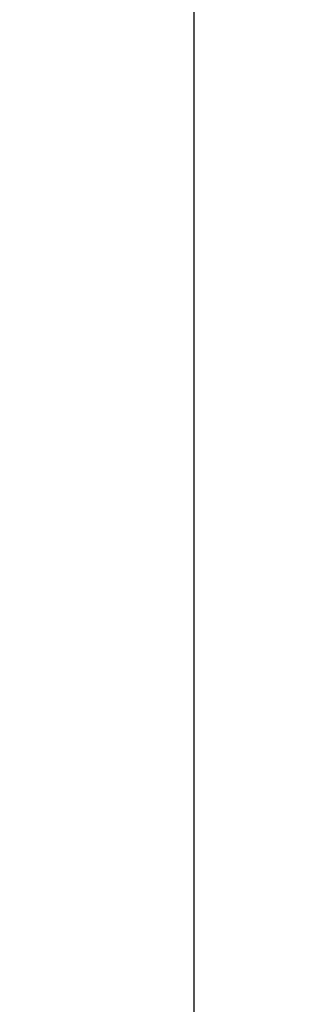
# Model space of a CAD drawing. Units: inches. Extents: x 2083 to 3317, y 1141 to 2115.
# Tile 75 of 256: x 2237.106 to 2238.294, y 1481.434 to 1485.751. Entities that reach past the tile are written whole.
import ezdxf

# ---------------------------------------------------------------- set-up
doc = ezdxf.new("R2010")
doc.units = ezdxf.units.IN
doc.layers.add('A-ANNO-DIMS', color=2, linetype='Continuous', lineweight=18)
doc.layers.add('A-WALL-PATT', color=251, linetype='Continuous', lineweight=13, true_color=0x636466)
doc.styles.get("Standard").update_dxf_attribs({"font": 'arial.ttf'})
doc.dimstyles.new('ISO-25', dxfattribs={"dimtxt": 12, "dimasz": 12, "dimexe": 1.25, "dimexo": 0.625, "dimtad": 1, "dimlunit": 3, "dimtxsty": 'Standard', "dimcen": 2.5, "dimadec": 0, "dimazin": 0, "dimtfac": 1, "dimtmove": 0, "dimatfit": 3, "dimfxl": 1, "dimarcsym": 0})

# ---------------------------------------------------------------- blocks, each defined once
blk = doc.blocks.new('*D30')
at = {"layer": 'A-ANNO-DIMS', "color": 0, "lineweight": -2, "transparency": 16777216}
for p, q in [((2240.0179, 1445.2738), (2240.0179, 1448.0455)), ((2254.3293, 1445.2738), (2254.3293, 1448.0455)), ((2228.0179, 1446.7955), (2216.0179, 1446.7955)), ((2240.0179, 1446.7955), (2254.3293, 1446.7955)), ((2266.3293, 1446.7955), (2413.7649, 1446.7955))]:
    blk.add_line(p, q, dxfattribs=at)
at = {"layer": 'A-ANNO-DIMS', "color": 0, "transparency": 16777216}
for points in [[(2228.0179, 1448.7955), (2228.0179, 1444.7955), (2240.0179, 1446.7955)], [(2266.3293, 1448.7955), (2266.3293, 1444.7955), (2254.3293, 1446.7955)]]:
    blk.add_solid(points, dxfattribs=at)
at = {"layer": 'Defpoints', "color": 0, "transparency": 16777216}
for p in [(2254.3293, 1446.7955), (2240.0179, 1444.6488), (2254.3293, 1444.6488)]:
    blk.add_point(p, dxfattribs=at)
at = {"layer": 'A-ANNO-DIMS', "color": 0, "transparency": 16777216, "insert": (2346.0471, 1453.6252), "char_height": 12, "attachment_point": 5}
blk.add_mtext('WC 1\'-2 1/2" TYP.', dxfattribs=at)
blk = doc.blocks.new('*D31')
at = {"layer": 'A-ANNO-DIMS', "color": 0, "lineweight": -2, "transparency": 16777216}
for p, q in [((2237.8711, 1456.6488), (2237.8711, 1541.9152)), ((2239.3929, 1444.6488), (2236.6211, 1444.6488)), ((2237.8711, 1431.5475), (2237.8711, 1444.6488)), ((2239.3929, 1431.5475), (2236.6211, 1431.5475)), ((2237.8711, 1419.5475), (2237.8711, 1407.5475))]:
    blk.add_line(p, q, dxfattribs=at)
at = {"layer": 'A-ANNO-DIMS', "color": 0, "transparency": 16777216}
for points in [[(2235.8711, 1456.6488), (2239.8711, 1456.6488), (2237.8711, 1444.6488)], [(2235.8711, 1419.5475), (2239.8711, 1419.5475), (2237.8711, 1431.5475)]]:
    blk.add_solid(points, dxfattribs=at)
at = {"layer": 'Defpoints', "color": 0, "transparency": 16777216}
for p in [(2237.8711, 1444.6488), (2240.0179, 1444.6488), (2240.0179, 1431.5475)]:
    blk.add_point(p, dxfattribs=at)
at = {"layer": 'A-ANNO-DIMS', "color": 0, "transparency": 16777216, "insert": (2231.2175, 1505.282), "char_height": 12, "attachment_point": 5, "rotation": 90}
blk.add_mtext('1\'-1" TYP.', dxfattribs=at)
blk = doc.blocks.new('*D45')
at = {"layer": 'A-ANNO-DIMS', "color": 0, "lineweight": -2, "transparency": 16777216}
for p, q in [((2235.9598, 1478.3864), (2235.9598, 1531.3614)), ((2418.9598, 1478.3864), (2418.9598, 1531.3614)), ((2247.9598, 1530.1114), (2406.9598, 1530.1114))]:
    blk.add_line(p, q, dxfattribs=at)
at = {"layer": 'A-ANNO-DIMS', "color": 0, "transparency": 16777216}
for points in [[(2247.9598, 1532.1114), (2247.9598, 1528.1114), (2235.9598, 1530.1114)], [(2406.9598, 1532.1114), (2406.9598, 1528.1114), (2418.9598, 1530.1114)]]:
    blk.add_solid(points, dxfattribs=at)
at = {"layer": 'Defpoints', "color": 0, "transparency": 16777216}
for p in [(2418.9598, 1530.1114), (2235.9598, 1477.7614), (2418.9598, 1477.7614)]:
    blk.add_point(p, dxfattribs=at)
at = {"layer": 'A-ANNO-DIMS', "color": 0, "transparency": 16777216, "insert": (2327.4598, 1536.8673), "char_height": 12, "attachment_point": 5}
blk.add_mtext('15\'-3"', dxfattribs=at)
blk = doc.blocks.new('*D62')
at = {"layer": 'A-ANNO-DIMS', "color": 0, "lineweight": -2, "transparency": 16777216}
for p, q in [((2235.9598, 1469.3864), (2235.9598, 1522.3614)), ((2379.9598, 1469.3864), (2379.9598, 1522.3614)), ((2247.9598, 1521.1114), (2367.9598, 1521.1114))]:
    blk.add_line(p, q, dxfattribs=at)
at = {"layer": 'A-ANNO-DIMS', "color": 0, "transparency": 16777216}
for points in [[(2247.9598, 1523.1114), (2247.9598, 1519.1114), (2235.9598, 1521.1114)], [(2367.9598, 1523.1114), (2367.9598, 1519.1114), (2379.9598, 1521.1114)]]:
    blk.add_solid(points, dxfattribs=at)
at = {"layer": 'Defpoints', "color": 0, "transparency": 16777216}
for p in [(2379.9598, 1521.1114), (2235.9598, 1468.7614), (2379.9598, 1468.7614)]:
    blk.add_point(p, dxfattribs=at)
at = {"layer": 'A-ANNO-DIMS', "color": 0, "transparency": 16777216, "insert": (2307.9598, 1527.8632), "char_height": 12, "attachment_point": 5}
blk.add_mtext('12\'-0"', dxfattribs=at)

msp = doc.modelspace()

# ---------------------------------------------------------------- hatches: boundary and pattern name
at = {"layer": 'A-WALL-PATT'}
h = msp.add_hatch(color=256, dxfattribs=at)
h.dxf.hatch_style = 1
h.paths.add_polyline_path([(3126.9598, 2020.7614), (2748.9598, 2020.7614), (2604.9598, 2020.7614), (2226.9598, 2020.7614), (2226.9598, 1702.7614), (2466.9598, 1702.7614), (2466.9598, 1582.7614), (2418.9598, 1582.7614), (2418.9598, 1477.7614), (2226.9598, 1477.7614), (2226.9598, 1263.2614), (2544.9598, 1263.2614), (2544.9598, 1411.7614), (2604.9598, 1411.7614), (2685.9598, 1411.7614), (2685.9598, 1420.7614), (2604.9598, 1420.7614), (2604.9598, 1573.7614), (2604.9598, 1702.7614), (2604.9598, 2011.7614), (2748.9598, 2011.7614), (2748.9598, 1702.7614), (2862.9598, 1702.7614), (2862.9598, 1621.7614), (2871.9598, 1621.7614), (2871.9598, 1702.7614), (2883.9598, 1702.7614), (2883.9598, 1706.9395, -0.026459), (2883.9598, 1711.7614), (2757.9598, 1711.7614), (2757.9598, 1807.7614), (2787.9598, 1807.7614), (2787.9598, 1812.2614), (2757.9598, 1812.2614), (2757.9598, 2011.7614), (2877.9598, 2011.7614), (2877.9598, 1812.2614), (2847.9598, 1812.2614), (2847.9598, 1807.7614), (2889.8357, 1807.7614), (2889.8357, 1812.2614), (2882.4598, 1812.2614), (2882.4598, 2011.7614), (3117.9598, 2011.7614), (3117.9598, 1812.2614), (2937.8357, 1812.2614), (2937.8357, 1807.7614), (2995.7098, 1807.7614), (2995.7098, 1796.1177), (3000.2098, 1796.1177), (3000.2098, 1807.7614), (3117.9598, 1807.7614), (3117.9598, 1711.7614), (3000.2098, 1711.7614), (3000.2098, 1760.1177), (2998.5727, 1760.1177, -0.020711), (2995.7098, 1760.1177), (2995.7098, 1711.7614), (2931.9598, 1711.7614), (2931.9598, 1702.7614), (3126.9598, 1702.7614)])
h.paths.add_polyline_path([(2471.4598, 2011.7614), (2471.4598, 1810.0114), (2462.7169, 1810.0114), (2462.7169, 1805.5114), (2505.9598, 1805.5114), (2505.9598, 1810.0114), (2475.9598, 1810.0114), (2475.9598, 2011.7614), (2595.9598, 2011.7614), (2595.9598, 1810.0114), (2565.9598, 1810.0114), (2565.9598, 1805.5114), (2595.9598, 1805.5114), (2595.9598, 1711.7614), (2235.9598, 1711.7614), (2235.9598, 1805.5114), (2353.7098, 1805.5114), (2353.7098, 1796.0542), (2358.2098, 1796.0542), (2358.2098, 1805.5114), (2414.7169, 1805.5114), (2414.7169, 1810.0114), (2235.9598, 1810.0114), (2235.9598, 2011.7614)], flags=16)
h.paths.add_polyline_path([(2270.2047, 1994.61), (2270.2047, 1970.61), (2246.2047, 1970.61), (2246.2047, 1994.61)], flags=0)
edge = h.paths.add_edge_path(flags=0)
edge.add_ellipse((2332.0274, 1899.7982), major_axis=(-3.043, 3.043), ratio=0.168252, start_angle=-161.3322, end_angle=-156.3071, ccw=False)
edge.add_ellipse((2333.082, 1898.7435), major_axis=(-1.0546, 1.0546), ratio=0.453532, start_angle=-123.371, end_angle=-94.1591)
edge = h.paths.add_edge_path(flags=0)
edge.add_ellipse((2332.0274, 1968.8763), major_axis=(3.043, 3.043), ratio=0.168252, start_angle=18.6678, end_angle=23.6929)
edge.add_spline(control_points=[(2332.9256, 1970.6911), (2332.2268, 1970.3361), (2330.8937, 1969.6589), (2328.4131, 1970.9321), (2327.2039, 1967.7487), (2324.7096, 1969.9556), (2322.5328, 1967.0124), (2320.0128, 1971.2958), (2317.6803, 1968.1578), (2316.0405, 1967.102), (2315.4269, 1966.8096)], knot_values=[0, 0, 0, 0, 2.267059, 4.324559, 6.685584, 8.878641, 11.121502, 14.300359, 17.755284, 19.732645, 19.732645, 19.732645, 19.732645], degree=3, periodic=0)
edge.add_ellipse((2332.0274, 1968.8763), major_axis=(3.043, 3.043), ratio=0.168252, start_angle=18.6678, end_angle=23.6929, ccw=False)
edge.add_ellipse((2333.082, 1969.9309), major_axis=(1.0546, 1.0546), ratio=0.453532, start_angle=56.629, end_angle=85.8409, ccw=False)
edge = h.paths.add_edge_path(flags=0)
edge.add_spline(control_points=[(2296.4283, 1967.9879), (2293.6278, 1965.3363), (2287.7036, 1959.7271), (2299.7439, 1949.9957), (2294.5326, 1935.6685), (2290.5732, 1920.6035), (2293.3941, 1909.9737), (2296.1854, 1904.9665)], knot_values=[0.099185, 0.099185, 0.099185, 0.099185, 0.345301, 0.619822, 0.982653, 1.386093, 1.810555, 1.810555, 1.810555, 1.810555], degree=3, periodic=0)
edge.add_spline(control_points=[(2296.1854, 1904.9665), (2297.3836, 1902.6193), (2298.001, 1901.9493), (2298.553, 1901.4682)], knot_values=[0.006246, 0.006246, 0.006246, 0.006246, 0.055476, 0.055476, 0.055476, 0.055476], degree=3, periodic=0)
edge.add_spline(control_points=[(2298.553, 1901.4682), (2297.2586, 1900.9232), (2295.2253, 1900.2321), (2293.0602, 1900.6142), (2292.1014, 1900.7884), (2292.0896, 1900.7906)], knot_values=[0.312835, 0.312835, 0.312835, 0.312835, 0.40178, 0.474987, 0.475903, 0.475903, 0.475903, 0.475903], degree=3, periodic=0)
edge.add_arc((2292.7936, 1904.6641), 3.937, 215.4209, 259.6982, ccw=False)
edge.add_spline(control_points=[(2289.5853, 1902.3823), (2289.4767, 1902.5351), (2289.3685, 1902.688), (2289.2609, 1902.8412)], knot_values=[0.102872, 0.102872, 0.102872, 0.102872, 0.116896, 0.116896, 0.116896, 0.116896], degree=3, periodic=0)
edge.add_spline(control_points=[(2289.2609, 1902.8412), (2288.6866, 1902.5502), (2287.64, 1902.0199), (2285.8813, 1901.874), (2283.853, 1901.5044), (2281.72, 1899.7105), (2278.467, 1899.4929), (2276.1571, 1901.8832), (2272.259, 1899.8041), (2267.7776, 1901.8432), (2262.2439, 1900.184), (2257.4149, 1901.7821), (2254.3184, 1900.7261), (2253.1783, 1900.3373)], knot_values=[0, 0, 0, 0, 1.907977, 3.477176, 5.261074, 7.972851, 11.680248, 13.717921, 16.939592, 22.789562, 27.502503, 33.595215, 37.145618, 37.145618, 37.145618, 37.145618], degree=3, periodic=0)
edge.add_line((2253.1783, 1900.3373), (2250.2442, 1902.8412))
edge.add_line((2250.2442, 1902.8412), (2250.2442, 1965.8333))
edge.add_line((2250.2442, 1965.8333), (2253.1783, 1968.3371))
edge.add_spline(control_points=[(2253.1783, 1968.3371), (2254.3184, 1967.9483), (2257.4149, 1966.8924), (2262.2439, 1968.4904), (2267.7776, 1966.8313), (2271.5267, 1968.5372), (2273.8759, 1967.8283), (2274.2067, 1967.7276)], knot_values=[0, 0, 0, 0, 0.09018, 0.244935, 0.364644, 0.513233, 0.537855, 0.537855, 0.537855, 0.537855], degree=3, periodic=0)
edge.add_arc((2274.3529, 1963.7933), 3.937, 72.0511, 92.1279, ccw=False)
edge.add_arc((2281.2969, 1985.23), 18.5963, 252.05113, 288.56572)
edge.add_arc((2292.3167, 1956.0289), 12.6461, 71.02679, 113.77822, ccw=False)
edge = h.paths.add_edge_path(flags=0)
edge.add_spline(control_points=[(2274.8994, 1951.8562), (2275.0662, 1951.6166), (2275.2327, 1951.3766), (2275.398, 1951.1359)], knot_values=[1.409916, 1.409916, 1.409916, 1.409916, 1.43159, 1.43159, 1.43159, 1.43159], degree=3, periodic=0)
edge.add_spline(control_points=[(2275.398, 1951.1359), (2275.7921, 1950.5619), (2276.1792, 1949.9838), (2276.5455, 1949.3971)], knot_values=[1.358238, 1.358238, 1.358238, 1.358238, 1.409916, 1.409916, 1.409916, 1.409916], degree=3, periodic=0)
edge.add_line((2276.5455, 1949.3971), (2277.4373, 1947.8622))
edge.add_spline(control_points=[(2277.4373, 1947.8622), (2276.3038, 1945.6731), (2274.6397, 1942.4269), (2274.6316, 1938.0939), (2272.7991, 1930.8515), (2274.3564, 1943.897), (2275.9477, 1947.9234), (2276.5455, 1949.3971)], knot_values=[0.005632, 0.005632, 0.005632, 0.005632, 0.186014, 0.266002, 0.357087, 0.59639, 0.739732, 0.739732, 0.739732, 0.739732], degree=3, periodic=0)
edge.add_spline(control_points=[(2276.5455, 1949.3971), (2276.1792, 1949.9838), (2275.7921, 1950.5619), (2275.398, 1951.1359)], knot_values=[1.358238, 1.358238, 1.358238, 1.358238, 1.409916, 1.409916, 1.409916, 1.409916], degree=3, periodic=0)
edge.add_spline(control_points=[(2275.398, 1951.1359), (2274.9425, 1950.0805), (2274.2078, 1948.0253), (2273.9346, 1944.8515), (2272.4685, 1937.6275), (2273.4662, 1945.6965), (2274.7006, 1951.0595), (2274.8994, 1951.8562)], knot_values=[0.104364, 0.104364, 0.104364, 0.104364, 0.189636, 0.269624, 0.36071, 0.600013, 0.644622, 0.644622, 0.644622, 0.644622], degree=3, periodic=0)
h.paths.add_polyline_path([(2269.1675, 1963.1276, -0.357527), (2268.1706, 1960.9764, -0.092561), (2268.1706, 1939.4363, -0.357527), (2269.1675, 1937.2851, -0.357527), (2267.0163, 1938.282, -0.164785), (2254.6856, 1938.282, -0.357527), (2252.5344, 1937.2851, -0.357527), (2253.5313, 1939.4363, -0.092561), (2253.5313, 1960.9764, -0.357527), (2252.5344, 1963.1276, -0.357527), (2254.6856, 1962.1307, -0.164785), (2267.0163, 1962.1307, -0.357527)], flags=0)
h.paths.add_polyline_path([(2248.8741, 1967.8018), (2248.8741, 1957.0277), (2249.4578, 1957.0277), (2249.4578, 1911.6468), (2248.8741, 1911.6468), (2248.8741, 1900.8727), (2246.5119, 1900.8727, 0.197327), (2244.1497, 1902.4569), (2244.1497, 1966.2176, 0.197327), (2246.5119, 1967.8018)], flags=0)
h.paths.add_polyline_path([(2269.1675, 1931.3893, -0.357527), (2268.1706, 1929.2381, -0.092561), (2268.1706, 1907.6981, -0.357527), (2269.1675, 1905.5469, -0.357527), (2267.0163, 1906.5438, -0.164785), (2254.6856, 1906.5438, -0.357527), (2252.5344, 1905.5469, -0.357527), (2253.5313, 1907.6981, -0.092561), (2253.5313, 1929.2381, -0.357527), (2252.5344, 1931.3893, -0.357527), (2254.6856, 1930.3925, -0.164785), (2267.0163, 1930.3925, -0.357527)], flags=0)
edge = h.paths.add_edge_path(flags=0)
edge.add_spline(control_points=[(2276.1969, 1906.7237), (2276.1681, 1909.0289), (2276.114, 1913.3719), (2270.5984, 1924.925), (2273.9052, 1919.0128), (2275.9217, 1916.2621), (2275.4746, 1912.4021), (2277.2579, 1910.3806), (2276.696, 1908.225), (2276.6462, 1906.813), (2276.6178, 1906.0084)], knot_values=[0, 0, 0, 0, 8.61026, 16.221274, 18.843057, 23.804898, 27.440828, 29.356102, 31.203478, 33.650687, 33.650687, 33.650687, 33.650687], degree=3, periodic=0)
edge.add_spline(control_points=[(2276.6178, 1906.0084), (2276.6233, 1905.6241), (2276.4977, 1904.6287), (2275.4418, 1903.8547), (2274.9373, 1903.0804), (2274.8591, 1902.8412)], knot_values=[0.156488, 0.156488, 0.156488, 0.156488, 0.184398, 0.231376, 0.250598, 0.250598, 0.250598, 0.250598], degree=3, periodic=0)
edge.add_line((2274.8591, 1902.8412), (2276.506, 1902.8412))
edge.add_spline(control_points=[(2276.506, 1902.8412), (2276.7883, 1903.0849), (2277.6651, 1904.1252), (2278.2495, 1904.3407), (2277.6539, 1908.5274), (2278.1557, 1906.2278), (2278.1005, 1905.2859), (2278.8467, 1904.069), (2277.8568, 1903.4149), (2277.8742, 1902.991), (2277.9036, 1902.8412)], knot_values=[0.059574, 0.059574, 0.059574, 0.059574, 0.080753, 0.103741, 0.16972, 0.176036, 0.207137, 0.240474, 0.262341, 0.27366, 0.27366, 0.27366, 0.27366], degree=3, periodic=0)
edge.add_line((2277.9036, 1902.8412), (2280.0298, 1902.8412))
edge.add_spline(control_points=[(2280.0298, 1902.8412), (2279.8882, 1903.0884), (2279.4993, 1903.9816), (2280.1523, 1905.9393), (2278.1036, 1909.6578), (2279.7624, 1907.1853), (2280.3279, 1904.8749), (2280.4851, 1903.4896), (2281.4633, 1903.2494), (2281.7583, 1902.9365), (2281.834, 1902.8412)], knot_values=[0.013856, 0.013856, 0.013856, 0.013856, 0.034874, 0.088867, 0.107879, 0.126738, 0.158714, 0.193757, 0.217487, 0.226722, 0.226722, 0.226722, 0.226722], degree=3, periodic=0)
edge.add_spline(control_points=[(2281.834, 1902.8412), (2281.7875, 1902.8267), (2281.647, 1902.783), (2281.3955, 1902.8595), (2281.0881, 1902.9852), (2280.7207, 1903.0609), (2280.3335, 1903.0257), (2280.1248, 1902.8989), (2280.0298, 1902.8412)], knot_values=[0, 0, 0, 0, 0.14413, 0.435517, 0.749276, 1.153046, 1.548371, 1.878348, 1.878348, 1.878348, 1.878348], degree=3, periodic=0)
edge.add_line((2280.0298, 1902.8412), (2277.9036, 1902.8412))
edge.add_spline(control_points=[(2277.9036, 1902.8412), (2277.8929, 1902.7959), (2277.8654, 1902.6796), (2277.6075, 1902.6875), (2277.2741, 1902.8007), (2276.8379, 1902.6198), (2276.5838, 1902.7893), (2276.506, 1902.8412)], knot_values=[0, 0, 0, 0, 0.127189, 0.326199, 0.628009, 1.24357, 1.515331, 1.515331, 1.515331, 1.515331], degree=3, periodic=0)
edge.add_line((2276.506, 1902.8412), (2274.8591, 1902.8412))
edge.add_spline(control_points=[(2274.8591, 1902.8412), (2274.8144, 1902.8986), (2274.7251, 1903.0134), (2274.4935, 1903.119), (2274.2443, 1902.9605), (2273.9371, 1903.1849), (2273.614, 1902.9831), (2273.4083, 1902.883), (2273.3223, 1902.8412)], knot_values=[0, 0, 0, 0, 0.21843, 0.436957, 0.687977, 0.990379, 1.398396, 1.69185, 1.69185, 1.69185, 1.69185], degree=3, periodic=0)
edge.add_spline(control_points=[(2273.3223, 1902.8412), (2273.6167, 1903.4457), (2274.274, 1904.5383), (2276.0272, 1904.5737), (2276.207, 1906.5836), (2276.1969, 1906.7237)], knot_values=[0.012227, 0.012227, 0.012227, 0.012227, 0.059472, 0.106218, 0.134458, 0.134458, 0.134458, 0.134458], degree=3, periodic=0)
h.paths.add_polyline_path([(2270.7761, 1897.7898), (2270.7761, 1873.7898), (2246.7761, 1873.7898), (2246.7761, 1897.7898)], flags=0)
h.paths.add_polyline_path([(2353.7098, 1760.0051), (2353.7098, 1760.0542), (2358.2098, 1760.0542, -0.033729)], flags=0)
h.paths.add_polyline_path([(2321.8191, 1737.5292), (2341.9953, 1737.5292, -0.414214), (2343.2033, 1736.3212), (2343.2033, 1721.0206, -0.414214), (2341.9953, 1719.8127), (2321.8191, 1719.8127, -0.414214), (2320.6112, 1721.0206), (2320.6112, 1736.3212, -0.414214)], flags=0)
h.paths.add_polyline_path([(2324.235, 1736.3212), (2339.5794, 1736.3212, -0.414214), (2341.9953, 1733.9053), (2341.9953, 1725.4497, -0.414214), (2339.5794, 1723.0338), (2333.6806, 1723.0338), (2333.8453, 1722.0455, -0.870646), (2335.4254, 1721.8259, -0.767327), (2333.9227, 1721.4232), (2331.291, 1721.4232, -0.767327), (2329.7883, 1721.8259, -0.870646), (2331.3684, 1722.0455), (2331.5331, 1723.0338), (2324.235, 1723.0338, -0.414214), (2321.8191, 1725.4497), (2321.8191, 1733.9053, -0.414214)], flags=0)
h.paths.add_polyline_path([(2570.4838, 1928.6154), (2589.6838, 1928.6154), (2590.1688, 1928.6154), (2590.1688, 1904.9934), (2570.4838, 1904.9934)], flags=0)
h.paths.add_polyline_path([(2574.4473, 1927.2638, -1), (2572.8288, 1927.2638, -1)], flags=0)
h.paths.add_polyline_path([(2573.0899, 1926.9409), (2573.925, 1927.776), (2574.1477, 1927.5533), (2573.3126, 1926.7182)], flags=0)
h.paths.add_polyline_path([(2578.7791, 1919.7296, -1), (2571.5917, 1919.7296, -1)], flags=0)
h.paths.add_polyline_path([(2578.3854, 1919.7296, -1), (2571.9854, 1919.7296, -1)], flags=0)
h.paths.add_polyline_path([(2331.5958, 1729.4762, -1), (2333.618, 1729.4762, -1)], flags=0)
h.paths.add_polyline_path([(2578.0342, 1927.2638, -1), (2576.4157, 1927.2638, -1)], flags=0)
h.paths.add_polyline_path([(2576.6889, 1927.5311), (2576.9116, 1927.7538), (2577.7467, 1926.9186), (2577.524, 1926.6959)], flags=0)
h.paths.add_polyline_path([(2578.1391, 1909.8595, -1), (2572.2317, 1909.8595, -1)], flags=0)
h.paths.add_polyline_path([(2577.7454, 1909.8595, -1), (2572.6254, 1909.8595, -1)], flags=0)
h.paths.add_polyline_path([(2583.7977, 1927.2638, -1), (2582.1792, 1927.2638, -1)], flags=0)
h.paths.add_polyline_path([(2582.7186, 1927.7538), (2583.5538, 1926.9186), (2583.3311, 1926.6959), (2582.4959, 1927.5311)], flags=0)
h.paths.add_polyline_path([(2582.4959, 1927.5311), (2582.7186, 1927.7538), (2583.5538, 1926.9186), (2583.3311, 1926.6959)], flags=0)
h.paths.add_polyline_path([(2587.7391, 1920.5296, -1), (2581.8317, 1920.5296, -1)], flags=0)
h.paths.add_polyline_path([(2587.3454, 1920.5296, -1), (2582.2254, 1920.5296, -1)], flags=0)
h.paths.add_polyline_path([(2587.3846, 1927.2638, -1), (2585.7661, 1927.2638, -1)], flags=0)
h.paths.add_polyline_path([(2586.082, 1926.9802), (2586.9172, 1927.8154), (2587.1399, 1927.5927), (2586.3047, 1926.7575)], flags=0)
h.paths.add_polyline_path([(2588.3791, 1910.6595, -1), (2581.1917, 1910.6595, -1)], flags=0)
h.paths.add_polyline_path([(2587.9854, 1910.6595, -1), (2581.5854, 1910.6595, -1)], flags=0)
h.paths.add_polyline_path([(2417.1677, 1729.4779), (2437.3439, 1729.4779, -0.414214), (2438.5519, 1728.2699), (2438.5519, 1712.9693, -0.414214), (2437.3439, 1711.7614), (2417.1677, 1711.7614, -0.414214), (2415.9598, 1712.9693), (2415.9598, 1728.2699, -0.414214)], flags=0)
h.paths.add_polyline_path([(2419.5836, 1728.2699), (2434.928, 1728.2699, -0.414214), (2437.3439, 1725.8541), (2437.3439, 1717.3984, -0.414214), (2434.928, 1714.9825), (2429.0292, 1714.9825), (2429.1939, 1713.9942, -0.870646), (2430.774, 1713.7746, -0.767327), (2429.2713, 1713.372), (2426.6396, 1713.372, -0.767327), (2425.1369, 1713.7746, -0.870646), (2426.717, 1713.9942), (2426.8817, 1714.9825), (2419.5836, 1714.9825, -0.414214), (2417.1677, 1717.3984), (2417.1677, 1725.8541, -0.414214)], flags=0)
h.paths.add_polyline_path([(2419.5836, 1728.2699), (2434.928, 1728.2699, -0.414214), (2437.3439, 1725.8541), (2437.3439, 1717.3984, -0.414214), (2434.928, 1714.9825), (2429.0292, 1714.9825), (2428.3581, 1719.009), (2427.5528, 1719.009), (2426.8817, 1714.9825), (2419.5836, 1714.9825, -0.414214), (2417.1677, 1717.3984), (2417.1677, 1725.8541, -0.414214)], flags=0)
h.paths.add_polyline_path([(2426.9444, 1721.4249, -1), (2428.9666, 1721.4249, -1)], flags=0)
h.paths.add_polyline_path([(2475.9598, 1702.7614), (2595.9598, 1702.7614), (2595.9598, 1582.7614), (2475.9598, 1582.7614)], flags=16)
h.paths.add_polyline_path([(2427.9598, 1573.7614), (2595.9598, 1573.7614), (2595.9598, 1468.7614), (2595.9598, 1420.7614), (2384.4598, 1420.7614), (2384.4598, 1468.7614), (2427.9598, 1468.7614)], flags=16)
h.paths.add_polyline_path([(2379.9598, 1468.7614), (2379.9598, 1420.7614), (2235.9598, 1420.7614), (2235.9598, 1468.7614)], flags=16)
h.paths.add_polyline_path([(2317.816, 1466.6958), (2337.9922, 1466.6958, -0.414214), (2339.2002, 1465.4878), (2339.2002, 1450.1872, -0.414214), (2337.9922, 1448.9792), (2317.816, 1448.9792, -0.414214), (2316.6081, 1450.1872), (2316.6081, 1465.4878, -0.414214)], flags=0)
h.paths.add_polyline_path([(2320.2319, 1465.4878), (2335.5763, 1465.4878, -0.414214), (2337.9922, 1463.0719), (2337.9922, 1454.6163, -0.414214), (2335.5763, 1452.2004), (2329.6775, 1452.2004), (2329.8422, 1451.212, -0.870646), (2331.4223, 1450.9925, -0.767327), (2329.9196, 1450.5898), (2327.2879, 1450.5898, -0.767327), (2325.7852, 1450.9925, -0.870646), (2327.3653, 1451.212), (2327.53, 1452.2004), (2320.2319, 1452.2004, -0.414214), (2317.816, 1454.6163), (2317.816, 1463.0719, -0.414214)], flags=0)
h.paths.add_polyline_path([(2320.2319, 1465.4878), (2335.5763, 1465.4878, -0.414214), (2337.9922, 1463.0719), (2337.9922, 1454.6163, -0.414214), (2335.5763, 1452.2004), (2329.6775, 1452.2004), (2329.0064, 1456.2269), (2328.2011, 1456.2269), (2327.53, 1452.2004), (2320.2319, 1452.2004, -0.414214), (2317.816, 1454.6163), (2317.816, 1463.0719, -0.414214)], flags=0)
h.paths.add_polyline_path([(2327.5926, 1458.6428, -1), (2329.6148, 1458.6428, -1)], flags=0)
h.paths.add_polyline_path([(2244.4117, 1433.3405), (2241.9209, 1433.3405, -0.414214), (2240.0179, 1435.2435), (2240.0179, 1440.9528, -0.414211), (2241.9209, 1442.8559), (2244.4117, 1442.8559, -1.976472)], flags=0)
h.paths.add_polyline_path([(2245.3569, 1434.3975, -0.414214), (2245.3569, 1441.7988, -2.144098)], flags=0)
h.paths.add_polyline_path([(2535.9598, 1416.2614), (2535.9598, 1272.2614), (2235.9598, 1272.2614), (2235.9598, 1416.2614)], flags=16)
h.paths.add_polyline_path([(2260.1196, 1384.2928), (2260.1196, 1362.0386), (2237.8654, 1362.0386), (2237.8654, 1384.2928)], flags=0)
edge = h.paths.add_edge_path(flags=0)
edge.add_line((2318.2518, 1362.0933), (2318.1458, 1362.001))
edge.add_ellipse((2317.4451, 1360.431), major_axis=(2.8216, 2.8216), ratio=0.168252, start_angle=18.6678, end_angle=20.9481, ccw=False)
edge.add_ellipse((2318.423, 1361.409), major_axis=(0.9779, 0.9779), ratio=0.453532, start_angle=56.629, end_angle=70.2262, ccw=False)
edge = h.paths.add_edge_path(flags=0)
edge.add_line((2319.1074, 1295.5711), (2319.015, 1295.6771))
edge.add_ellipse((2317.4451, 1296.3778), major_axis=(-2.8216, 2.8216), ratio=0.168252, start_angle=-161.3322, end_angle=-159.0519, ccw=False)
edge.add_ellipse((2318.423, 1295.3999), major_axis=(-0.9779, 0.9779), ratio=0.453532, start_angle=-123.371, end_angle=-109.7738)
edge = h.paths.add_edge_path(flags=0)
edge.add_spline(control_points=[(2284.2103, 1301.1702), (2284.5807, 1300.4447), (2284.8912, 1299.892), (2285.1596, 1299.461)], knot_values=[0.039066, 0.039066, 0.039066, 0.039066, 0.055476, 0.055476, 0.055476, 0.055476], degree=3, periodic=0)
edge.add_line((2285.1596, 1299.461), (2284.2103, 1301.1702))
edge = h.paths.add_edge_path(flags=0)
edge.add_line((2280.4125, 1297.298), (2283.37, 1297.0361))
edge.add_line((2283.37, 1297.0361), (2286.4057, 1297.9263))
edge.add_spline(control_points=[(2286.4057, 1297.9263), (2285.3055, 1297.4631), (2284.3448, 1297.1292), (2283.37, 1297.0361)], knot_values=[0.394369, 0.394369, 0.394369, 0.394369, 0.475903, 0.475903, 0.475903, 0.475903], degree=3, periodic=0)
edge.add_spline(control_points=[(2283.37, 1297.0361), (2283.2814, 1297.0277), (2282.3163, 1296.9573), (2281.3125, 1297.1345), (2280.4234, 1297.296), (2280.4125, 1297.298)], knot_values=[0.312835, 0.312835, 0.312835, 0.312835, 0.320246, 0.393453, 0.394369, 0.394369, 0.394369, 0.394369], degree=3, periodic=0)
edge = h.paths.add_edge_path(flags=0)
edge.add_line((2284.4356, 1359.6073), (2280.4463, 1355.328))
edge.add_line((2280.4463, 1355.328), (2279.58, 1351.0178))
edge.add_line((2279.58, 1351.0178), (2282.413, 1346.5804))
edge.add_spline(control_points=[(2282.413, 1346.5804), (2283.1533, 1345.5892), (2284.2529, 1344.0289), (2284.801, 1342.3872), (2284.9352, 1341.8055)], knot_values=[1.240098, 1.240098, 1.240098, 1.240098, 1.332892, 1.382712, 1.382712, 1.382712, 1.382712], degree=3, periodic=0)
edge.add_spline(control_points=[(2284.9352, 1341.8055), (2285.3191, 1340.1406), (2285.233, 1338.4092), (2284.9099, 1336.6541)], knot_values=[1.097484, 1.097484, 1.097484, 1.097484, 1.240098, 1.240098, 1.240098, 1.240098], degree=3, periodic=0)
edge.add_spline(control_points=[(2284.9099, 1336.6541), (2284.5868, 1334.899), (2284.0267, 1333.1203), (2283.4626, 1331.3606)], knot_values=[0.95487, 0.95487, 0.95487, 0.95487, 1.097484, 1.097484, 1.097484, 1.097484], degree=3, periodic=0)
edge.add_line((2283.4626, 1331.3606), (2281.8904, 1326.1534))
edge.add_line((2281.8904, 1326.1534), (2280.7563, 1321.0561))
edge.add_line((2280.7563, 1321.0561), (2280.2992, 1316.002))
edge.add_line((2280.2992, 1316.002), (2280.7159, 1310.9501))
edge.add_line((2280.7159, 1310.9501), (2282.0281, 1305.9721))
edge.add_line((2282.0281, 1305.9721), (2284.2103, 1301.1702))
edge.add_spline(control_points=[(2284.2103, 1301.1702), (2283.3407, 1302.7302), (2282.6119, 1304.3365), (2282.0281, 1305.9721)], knot_values=[0.099185, 0.099185, 0.099185, 0.099185, 0.241799, 0.241799, 0.241799, 0.241799], degree=3, periodic=0)
edge.add_spline(control_points=[(2282.0281, 1305.9721), (2281.4443, 1307.6078), (2281.0055, 1309.2728), (2280.7159, 1310.9501)], knot_values=[0.241799, 0.241799, 0.241799, 0.241799, 0.384413, 0.384413, 0.384413, 0.384413], degree=3, periodic=0)
edge.add_spline(control_points=[(2280.7159, 1310.9501), (2280.4332, 1312.5876), (2280.2894, 1314.277), (2280.2989, 1315.962), (2280.2992, 1316.002)], knot_values=[0.384413, 0.384413, 0.384413, 0.384413, 0.523647, 0.527028, 0.527028, 0.527028, 0.527028], degree=3, periodic=0)
edge.add_spline(control_points=[(2280.2992, 1316.002), (2280.3123, 1317.687), (2280.4779, 1319.3679), (2280.7563, 1321.0561)], knot_values=[0.527028, 0.527028, 0.527028, 0.527028, 0.669642, 0.669642, 0.669642, 0.669642], degree=3, periodic=0)
edge.add_spline(control_points=[(2280.7563, 1321.0561), (2281.0346, 1322.7443), (2281.4259, 1324.4396), (2281.8904, 1326.1534)], knot_values=[0.669642, 0.669642, 0.669642, 0.669642, 0.812256, 0.812256, 0.812256, 0.812256], degree=3, periodic=0)
edge.add_spline(control_points=[(2281.8904, 1326.1534), (2282.2644, 1327.5333), (2282.7879, 1329.2618), (2283.3528, 1331.0178), (2283.4626, 1331.3606)], knot_values=[0.812256, 0.812256, 0.812256, 0.812256, 0.927087, 0.95487, 0.95487, 0.95487, 0.95487], degree=3, periodic=0)
edge.add_line((2283.4626, 1331.3606), (2284.9099, 1336.6541))
edge.add_line((2284.9099, 1336.6541), (2284.9352, 1341.8055))
edge.add_line((2284.9352, 1341.8055), (2282.413, 1346.5804))
edge.add_spline(control_points=[(2282.413, 1346.5804), (2281.2751, 1348.1038), (2280.0784, 1349.5703), (2279.58, 1351.0178)], knot_values=[1.382712, 1.382712, 1.382712, 1.382712, 1.525326, 1.525326, 1.525326, 1.525326], degree=3, periodic=0)
edge.add_spline(control_points=[(2279.58, 1351.0178), (2279.4433, 1351.4147), (2279.1363, 1352.8569), (2279.7352, 1354.2904), (2280.4463, 1355.328)], knot_values=[1.525326, 1.525326, 1.525326, 1.525326, 1.564439, 1.667941, 1.667941, 1.667941, 1.667941], degree=3, periodic=0)
edge.add_spline(control_points=[(2280.4463, 1355.328), (2281.4261, 1356.7578), (2282.9308, 1358.1826), (2284.4356, 1359.6073)], knot_values=[1.667941, 1.667941, 1.667941, 1.667941, 1.810555, 1.810555, 1.810555, 1.810555], degree=3, periodic=0)
edge.add_arc((2280.6231, 1348.5182), 11.7262, 71.02679, 113.77822)
edge.add_arc((2270.4049, 1375.5952), 17.2436, 252.05113, 288.56572, ccw=False)
edge.add_arc((2263.966, 1355.7178), 3.6506, 72.0511, 92.1279)
edge.add_arc((2263.966, 1355.7178), 3.6506, 92.1279, 177.9851)
edge.add_spline(control_points=[(2260.3176, 1355.8462), (2260.2604, 1354.2207), (2260.5513, 1350.1865), (2262.9993, 1346.7663), (2264.4727, 1344.649)], knot_values=[1.43159, 1.43159, 1.43159, 1.43159, 1.564144, 1.770695, 1.770695, 1.770695, 1.770695], degree=3, periodic=0)
edge.add_line((2264.4727, 1344.649), (2264.9356, 1343.9825))
edge.add_spline(control_points=[(2263.801, 1340.2481), (2263.8432, 1340.5141), (2264.0672, 1341.7565), (2264.5127, 1343.0025), (2264.935, 1343.9811)], knot_values=[0.53657, 0.53657, 0.53657, 0.53657, 0.559349, 0.644622, 0.644622, 0.644622, 0.644622], degree=3, periodic=0)
edge.add_spline(control_points=[(2264.935, 1343.9811), (2265.1178, 1343.715), (2265.2989, 1343.4479), (2265.4768, 1343.1794)], knot_values=[1.384077, 1.384077, 1.384077, 1.384077, 1.409916, 1.409916, 1.409916, 1.409916], degree=3, periodic=0)
edge.add_spline(control_points=[(2265.4768, 1343.1794), (2265.6546, 1342.9108), (2265.8293, 1342.6408), (2265.9991, 1342.3688)], knot_values=[1.358238, 1.358238, 1.358238, 1.358238, 1.384077, 1.384077, 1.384077, 1.384077], degree=3, periodic=0)
edge.add_line((2265.9991, 1342.3688), (2266.826, 1340.9455))
edge.add_spline(control_points=[(2266.826, 1340.9455), (2268.8944, 1337.0897), (2271.3982, 1325.843), (2270.5162, 1310.5686), (2275.9194, 1301.8606), (2277.7895, 1299.1994)], knot_values=[0.116896, 0.116896, 0.116896, 0.116896, 0.472987, 1.050969, 1.313793, 1.313793, 1.313793, 1.313793], degree=3, periodic=0)
edge.add_spline(control_points=[(2277.7895, 1299.1994), (2277.8394, 1299.1285), (2277.8894, 1299.0575), (2277.9396, 1298.9866)], knot_values=[0.109884, 0.109884, 0.109884, 0.109884, 0.116896, 0.116896, 0.116896, 0.116896], degree=3, periodic=0)
edge.add_line((2277.9396, 1298.9866), (2277.7888, 1299.1991))
edge.add_spline(control_points=[(2277.7888, 1299.1991), (2277.2566, 1298.9294), (2276.2864, 1298.4379), (2275.0394, 1298.3344), (2274.3833, 1298.2389), (2274.2153, 1298.2093)], knot_values=[33.12187, 33.12187, 33.12187, 33.12187, 35.029056, 36.598255, 37.144827, 37.144827, 37.144827, 37.144827], degree=3, periodic=0)
edge.add_line((2274.2153, 1298.2093), (2273.0731, 1297.893))
edge.add_spline(control_points=[(2273.0731, 1297.893), (2272.3229, 1297.5798), (2271.0392, 1296.5105), (2269.2484, 1296.2261), (2268.4231, 1296.3747)], knot_values=[26.532584, 26.532584, 26.532584, 26.532584, 29.198919, 31.839101, 31.839101, 31.839101, 31.839101], degree=3, periodic=0)
edge.add_line((2268.4231, 1296.3747), (2263.8785, 1297.4575))
edge.add_spline(control_points=[(2263.8785, 1297.4575), (2263.5561, 1297.3594), (2261.8603, 1296.8387), (2260.2388, 1297.2824), (2258.9335, 1297.5165)], knot_values=[15.919551, 15.919551, 15.919551, 15.919551, 16.939592, 21.226067, 21.226067, 21.226067, 21.226067], degree=3, periodic=0)
edge.add_line((2258.9335, 1297.5165), (2254.0552, 1297.329))
edge.add_spline(control_points=[(2254.0552, 1297.329), (2253.7555, 1297.2958), (2252.1137, 1297.1652), (2250.4619, 1297.5442), (2249.1297, 1297.6679)], knot_values=[5.306517, 5.306517, 5.306517, 5.306517, 6.276435, 10.613034, 10.613034, 10.613034, 10.613034], degree=3, periodic=0)
edge.add_line((2249.1297, 1297.6679), (2244.3316, 1296.8778))
edge.add_line((2244.3316, 1296.8778), (2241.611, 1299.1994))
edge.add_line((2241.611, 1299.1994), (2241.611, 1357.6094))
edge.add_line((2241.611, 1357.6094), (2244.3316, 1359.9311))
edge.add_line((2244.3316, 1359.9311), (2252.7288, 1359.5427))
edge.add_spline(control_points=[(2252.7288, 1359.5427), (2252.8709, 1359.5464), (2253.3057, 1359.5482), (2253.7398, 1359.5143), (2254.0317, 1359.4824)], knot_values=[0.233291, 0.233291, 0.233291, 0.233291, 0.244935, 0.268927, 0.268927, 0.268927, 0.268927], degree=3, periodic=0)
edge.add_line((2254.0317, 1359.4824), (2259.5872, 1359.4164))
edge.add_spline(control_points=[(2259.5872, 1359.4164), (2260.6771, 1359.6285), (2262.0732, 1359.897), (2263.5237, 1359.4593), (2263.8304, 1359.366)], knot_values=[0.422516, 0.422516, 0.422516, 0.422516, 0.513233, 0.537855, 0.537855, 0.537855, 0.537855], degree=3, periodic=0)
edge.add_arc((2263.966, 1355.7178), 3.6506, 72.0511, 92.1279, ccw=False)
edge.add_arc((2270.4049, 1375.5952), 17.2436, 252.05113, 288.56572)
edge.add_arc((2280.6231, 1348.5182), 11.7262, 71.02679, 113.77822, ccw=False)
h.paths.add_polyline_path([(2240.3405, 1359.4347), (2240.3405, 1349.4444), (2240.8818, 1349.4444), (2240.8818, 1307.3645), (2240.3405, 1307.3645), (2240.3405, 1297.3741), (2238.1502, 1297.3741, 0.197327), (2235.9598, 1298.8431), (2235.9598, 1357.9657, 0.197327), (2238.1502, 1359.4347)], flags=0)
h.paths.add_polyline_path([(2259.1578, 1355.1005, -0.357527), (2258.2334, 1353.1058, -0.092561), (2258.2334, 1333.1326, -0.357527), (2259.1578, 1331.1379, -0.357527), (2257.1631, 1332.0622, -0.164785), (2245.7293, 1332.0622, -0.357527), (2243.7346, 1331.1379, -0.357527), (2244.6589, 1333.1326, -0.092561), (2244.6589, 1353.1058, -0.357527), (2243.7346, 1355.1005, -0.357527), (2245.7293, 1354.1761, -0.164785), (2257.1631, 1354.1761, -0.357527)], flags=0)
edge = h.paths.add_edge_path(flags=0)
edge.add_line((2265.9991, 1342.3688), (2266.826, 1340.9455))
edge.add_line((2266.826, 1340.9455), (2265.3076, 1337.8141))
edge.add_line((2265.3076, 1337.8141), (2264.3582, 1334.6529))
edge.add_line((2264.3582, 1334.6529), (2264.262, 1333.7997))
edge.add_spline(control_points=[(2264.262, 1333.7997), (2264.2084, 1333.1871), (2264.1621, 1332.3655), (2264.0071, 1331.4139), (2263.969, 1331.2018)], knot_values=[0.464444, 0.464444, 0.464444, 0.464444, 0.516691, 0.531608, 0.531608, 0.531608, 0.531608], degree=3, periodic=0)
edge.add_spline(control_points=[(2263.969, 1331.2018), (2263.7745, 1330.1189), (2263.4244, 1328.7908), (2263.2574, 1328.5307), (2263.234, 1328.5146)], knot_values=[0.372682, 0.372682, 0.372682, 0.372682, 0.44885, 0.464444, 0.464444, 0.464444, 0.464444], degree=3, periodic=0)
edge.add_spline(control_points=[(2263.234, 1328.5146), (2263.0964, 1328.4202), (2263.1312, 1329.3015), (2263.275, 1330.6157)], knot_values=[0.280919, 0.280919, 0.280919, 0.280919, 0.372682, 0.372682, 0.372682, 0.372682], degree=3, periodic=0)
edge.add_spline(control_points=[(2263.275, 1330.6157), (2263.4187, 1331.93), (2263.6715, 1333.6773), (2263.9699, 1335.315)], knot_values=[0.189157, 0.189157, 0.189157, 0.189157, 0.280919, 0.280919, 0.280919, 0.280919], degree=3, periodic=0)
edge.add_spline(control_points=[(2263.9699, 1335.315), (2264.1005, 1336.0322), (2264.4188, 1337.6219), (2264.7548, 1338.8644), (2264.9474, 1339.4911)], knot_values=[0.097394, 0.097394, 0.097394, 0.097394, 0.137578, 0.189157, 0.189157, 0.189157, 0.189157], degree=3, periodic=0)
edge.add_spline(control_points=[(2264.9474, 1339.4911), (2265.29, 1340.6061), (2265.6442, 1341.494), (2265.9991, 1342.3688)], knot_values=[0.005632, 0.005632, 0.005632, 0.005632, 0.097394, 0.097394, 0.097394, 0.097394], degree=3, periodic=0)
h.paths.add_polyline_path([(2259.1578, 1325.671, -0.357527), (2258.2334, 1323.6763, -0.092561), (2258.2334, 1303.7031, -0.357527), (2259.1578, 1301.7084, -0.357527), (2257.1631, 1302.6327, -0.164785), (2245.7293, 1302.6327, -0.357527), (2243.7346, 1301.7084, -0.357527), (2244.6589, 1303.7031, -0.092561), (2244.6589, 1323.6763, -0.357527), (2243.7346, 1325.671, -0.357527), (2245.7293, 1324.7466, -0.164785), (2257.1631, 1324.7466, -0.357527)], flags=0)
edge = h.paths.add_edge_path(flags=0)
edge.add_spline(control_points=[(2261.7089, 1317.3114), (2261.6795, 1317.4176), (2261.7619, 1317.3885), (2262.4907, 1316.0899), (2262.9622, 1315.3009)], knot_values=[14.955861, 14.955861, 14.955861, 14.955861, 16.221274, 18.694826, 18.694826, 18.694826, 18.694826], degree=3, periodic=0)
edge.add_spline(control_points=[(2262.9622, 1315.3009), (2262.9904, 1315.2536), (2263.7021, 1314.0674), (2264.349, 1313.1272), (2264.7301, 1312.1642)], knot_values=[18.694826, 18.694826, 18.694826, 18.694826, 18.843057, 22.433791, 22.433791, 22.433791, 22.433791], degree=3, periodic=0)
edge.add_spline(control_points=[(2264.7301, 1312.1642), (2264.8756, 1311.7964), (2265.1769, 1310.7698), (2265.1431, 1309.5593), (2265.2477, 1308.8242)], knot_values=[22.433791, 22.433791, 22.433791, 22.433791, 23.804898, 26.172756, 26.172756, 26.172756, 26.172756], degree=3, periodic=0)
edge.add_line((2265.2477, 1308.8242), (2265.8508, 1307.1719))
edge.add_spline(control_points=[(2265.8508, 1307.1719), (2266.065, 1306.8217), (2266.3844, 1306.3322), (2266.4244, 1305.7805), (2266.4204, 1305.6112)], knot_values=[28.062562, 28.062562, 28.062562, 28.062562, 29.356102, 29.911721, 29.911721, 29.911721, 29.911721], degree=3, periodic=0)
edge.add_spline(control_points=[(2266.4204, 1305.6112), (2266.4161, 1305.4326), (2266.394, 1305.25), (2266.3648, 1305.0659)], knot_values=[29.911721, 29.911721, 29.911721, 29.911721, 30.497837, 30.497837, 30.497837, 30.497837], degree=3, periodic=0)
edge.add_line((2266.3648, 1305.0659), (2266.0662, 1302.1363))
edge.add_spline(control_points=[(2266.0662, 1302.1363), (2266.0712, 1301.78), (2265.9981, 1301.2), (2265.6633, 1300.759), (2265.5089, 1300.5859)], knot_values=[0.156488, 0.156488, 0.156488, 0.156488, 0.184398, 0.203543, 0.203543, 0.203543, 0.203543], degree=3, periodic=0)
edge.add_line((2265.5089, 1300.5859), (2264.4353, 1299.1994))
edge.add_line((2264.4353, 1299.1994), (2265.9624, 1299.1994))
edge.add_line((2265.9624, 1299.1994), (2267.336, 1301.1753))
edge.add_line((2267.336, 1301.1753), (2267.3117, 1301.9862))
edge.add_spline(control_points=[(2267.3117, 1301.9862), (2267.2611, 1302.8624), (2267.1602, 1303.7371), (2267.2715, 1303.3259)], knot_values=[0.126229, 0.126229, 0.126229, 0.126229, 0.166617, 0.166617, 0.166617, 0.166617], degree=3, periodic=0)
edge.add_spline(control_points=[(2267.2715, 1303.3259), (2267.28, 1303.2943), (2267.3098, 1303.1754), (2267.3735, 1302.8836), (2267.4061, 1302.6828), (2267.4179, 1302.601)], knot_values=[0.166617, 0.166617, 0.166617, 0.166617, 0.16972, 0.176036, 0.180765, 0.180765, 0.180765, 0.180765], degree=3, periodic=0)
edge.add_spline(control_points=[(2267.7439, 1300.9875), (2267.6876, 1301.1509), (2267.4805, 1301.6567), (2267.4838, 1302.1448), (2267.4179, 1302.601)], knot_values=[0.180765, 0.180765, 0.180765, 0.180765, 0.193767, 0.220139, 0.220139, 0.220139, 0.220139], degree=3, periodic=0)
edge.add_line((2267.4179, 1302.601), (2267.7439, 1300.9875))
edge.add_spline(control_points=[(2267.7439, 1300.9875), (2267.832, 1300.7319), (2267.932, 1300.3099), (2267.5548, 1299.9745), (2267.4294, 1299.8292)], knot_values=[0.220139, 0.220139, 0.220139, 0.220139, 0.240474, 0.25489, 0.25489, 0.25489, 0.25489], degree=3, periodic=0)
edge.add_line((2267.4294, 1299.8292), (2267.2584, 1299.1994))
edge.add_line((2267.2584, 1299.1994), (2269.23, 1299.1994))
edge.add_spline(control_points=[(2269.23, 1299.1994), (2269.0987, 1299.4287), (2268.8428, 1300.0163), (2269.0116, 1300.9159), (2268.9468, 1301.6607)], knot_values=[0.013856, 0.013856, 0.013856, 0.013856, 0.034874, 0.067073, 0.067073, 0.067073, 0.067073], degree=3, periodic=0)
edge.add_line((2268.9468, 1301.6607), (2268.4316, 1303.6031))
edge.add_spline(control_points=[(2268.4316, 1303.6031), (2268.1756, 1304.1924), (2267.5962, 1305.2513), (2268.0407, 1304.6232), (2268.2514, 1304.2824)], knot_values=[0.090155, 0.090155, 0.090155, 0.090155, 0.107879, 0.120289, 0.120289, 0.120289, 0.120289], degree=3, periodic=0)
edge.add_spline(control_points=[(2268.2514, 1304.2824), (2268.3609, 1304.1053), (2269.0578, 1302.918), (2269.3827, 1301.5904), (2269.5214, 1300.7759), (2269.5752, 1300.5558)], knot_values=[0.120289, 0.120289, 0.120289, 0.120289, 0.126738, 0.158714, 0.173506, 0.173506, 0.173506, 0.173506], degree=3, periodic=0)
edge.add_line((2269.5752, 1300.5558), (2270.6858, 1299.4213))
edge.add_spline(control_points=[(2270.6858, 1299.4213), (2270.7672, 1299.3573), (2270.8379, 1299.2814), (2270.9029, 1299.1994)], knot_values=[0.21816, 0.21816, 0.21816, 0.21816, 0.226722, 0.226722, 0.226722, 0.226722], degree=3, periodic=0)
edge.add_line((2270.9372, 1299.1929), (2270.9029, 1299.1994))
edge.add_spline(control_points=[(2270.9029, 1299.1994), (2270.8598, 1299.186), (2270.7295, 1299.1455), (2270.4963, 1299.2164), (2270.2717, 1299.3083), (2270.121, 1299.348), (2270.0633, 1299.3596)], knot_values=[0.939174, 0.939174, 0.939174, 0.939174, 1.083304, 1.374691, 1.68845, 1.878348, 1.878348, 1.878348, 1.878348], degree=3, periodic=0)
edge.add_line((2270.0633, 1299.3596), (2269.23, 1299.1994))
edge.add_line((2269.23, 1299.1994), (2267.2584, 1299.1994))
edge.add_spline(control_points=[(2267.2584, 1299.1994), (2267.2484, 1299.1574), (2267.223, 1299.0497), (2266.9838, 1299.0569), (2266.8092, 1299.1162), (2266.6769, 1299.1091), (2266.6365, 1299.1048)], knot_values=[0.757665, 0.757665, 0.757665, 0.757665, 0.884854, 1.083864, 1.385675, 1.515331, 1.515331, 1.515331, 1.515331], degree=3, periodic=0)
edge.add_spline(control_points=[(2266.6365, 1299.1048), (2266.4852, 1299.0888), (2266.2358, 1299.0171), (2266.0346, 1299.1513), (2265.9624, 1299.1994)], knot_values=[0, 0, 0, 0, 0.485905, 0.757665, 0.757665, 0.757665, 0.757665], degree=3, periodic=0)
edge.add_line((2265.9624, 1299.1994), (2264.4353, 1299.1994))
edge.add_line((2264.4353, 1299.1994), (2263.8584, 1299.3671))
edge.add_spline(control_points=[(2263.8584, 1299.3671), (2263.8189, 1299.3709), (2263.7795, 1299.3857), (2263.7401, 1299.4015)], knot_values=[0.845925, 0.845925, 0.845925, 0.845925, 0.978627, 0.978627, 0.978627, 0.978627], degree=3, periodic=0)
edge.add_line((2263.7218, 1299.3964), (2263.0103, 1299.1994))
edge.add_spline(control_points=[(2263.0103, 1299.1994), (2263.2458, 1299.6829), (2263.506, 1300.1281), (2263.8735, 1300.408)], knot_values=[0.012227, 0.012227, 0.012227, 0.012227, 0.052971, 0.052971, 0.052971, 0.052971], degree=3, periodic=0)
edge.add_spline(control_points=[(2263.8735, 1300.408), (2263.9321, 1300.4527), (2264.0842, 1300.553), (2264.2552, 1300.6242), (2264.3597, 1300.6647)], knot_values=[0.052971, 0.052971, 0.052971, 0.052971, 0.059472, 0.069086, 0.069086, 0.069086, 0.069086], degree=3, periodic=0)
edge.add_line((2264.3597, 1300.6647), (2265.1419, 1301.0778))
edge.add_line((2265.1419, 1301.0778), (2265.6758, 1302.7996))
edge.add_line((2265.6758, 1302.7996), (2265.5407, 1305.7041))
edge.add_line((2265.5407, 1305.7041), (2264.8031, 1309.3277))
edge.add_line((2264.8031, 1309.3277), (2263.0405, 1314.0918))
edge.add_spline(control_points=[(2263.0405, 1314.0918), (2262.3836, 1315.6714), (2261.796, 1316.9977), (2261.7089, 1317.3114)], knot_values=[11.216896, 11.216896, 11.216896, 11.216896, 14.955861, 14.955861, 14.955861, 14.955861], degree=3, periodic=0)
h.paths.add_polyline_path([(2871.9598, 1416.2614), (2895.91, 1416.2614), (2895.91, 1420.7614), (2871.9598, 1420.7614), (2871.9598, 1501.7614), (2862.9598, 1501.7614), (2862.9598, 1420.7614), (2805.9598, 1420.7614), (2805.9598, 1411.7614), (2862.9598, 1411.7614), (2862.9598, 1263.2614), (3126.9598, 1263.2614), (3126.9598, 1411.7614), (3126.9598, 1486.7614), (2943.9598, 1486.7614), (2943.9598, 1477.7614), (2967.8603, 1477.7614), (2967.8603, 1420.7614), (2943.91, 1420.7614), (2943.91, 1416.2614), (3117.9598, 1416.2614), (3117.9598, 1420.7614), (2972.3603, 1420.7614), (2972.3603, 1477.7614), (3117.9598, 1477.7614), (3117.9598, 1420.7614), (3117.9598, 1272.2614), (2871.9598, 1272.2614)], flags=0)
h.paths.add_polyline_path([(2457.1256, 1485.9425), (2527.6027, 1485.9425), (2527.6027, 1537.6357), (2457.1256, 1537.6357)], flags=8)
h.paths.add_polyline_path([(2481.0051, 1609.9818), (2590.7658, 1609.9818), (2590.7658, 1682.0034), (2481.0051, 1682.0034)], flags=8)
h.paths.add_polyline_path([(2483.085, 1729.1268), (2553.562, 1729.1268), (2553.562, 1780.82), (2483.085, 1780.82)], flags=8)

# ---------------------------------------------------------------- dimensions: what is measured, and where the dimension line sits
at = {"layer": 'A-ANNO-DIMS'}
for base, p1, p2, picture, middle in [((2418.9598, 1530.1114), (2235.9598, 1477.7614), (2418.9598, 1477.7614), '*D45', (2327.4598, 1536.8673)), ((2379.9598, 1521.1114), (2235.9598, 1468.7614), (2379.9598, 1468.7614), '*D62', (2307.9598, 1527.8632))]:
    dim = msp.add_linear_dim(base=base, p1=p1, p2=p2, dimstyle='ISO-25', override={"dimdec": 1, "dimlfac": 1, "dimrnd": 0, "dimzin": 1, "dimdsep": 46, "dimlunit": 4, "dimfrac": 2}, dxfattribs=at)
    dim.commit()
    dim.dimension.update_dxf_attribs({"geometry": picture, "text_midpoint": middle})
dim = msp.add_linear_dim(base=(2237.8711, 1444.6488), p1=(2240.0179, 1431.5475), p2=(2240.0179, 1444.6488), angle=90, text='<> TYP.', dimstyle='ISO-25', override={"dimdec": 1, "dimlfac": 1, "dimrnd": 0, "dimzin": 1, "dimdsep": 46, "dimlunit": 4, "dimfrac": 2}, dxfattribs=at)
dim.commit()
dim.dimension.update_dxf_attribs({"geometry": '*D31', "text_midpoint": (2231.2175, 1505.282)})
dim = msp.add_linear_dim(base=(2254.3293, 1446.7955), p1=(2240.0179, 1444.6488), p2=(2254.3293, 1444.6488), text='WC <> TYP.', dimstyle='ISO-25', override={"dimdec": 1, "dimlfac": 1, "dimrnd": 0, "dimzin": 1, "dimdsep": 46, "dimlunit": 4, "dimfrac": 2}, dxfattribs=at)
dim.commit()
dim.dimension.update_dxf_attribs({"geometry": '*D30', "text_midpoint": (2346.0471, 1453.6252)})

doc.saveas('drawing.dxf')
